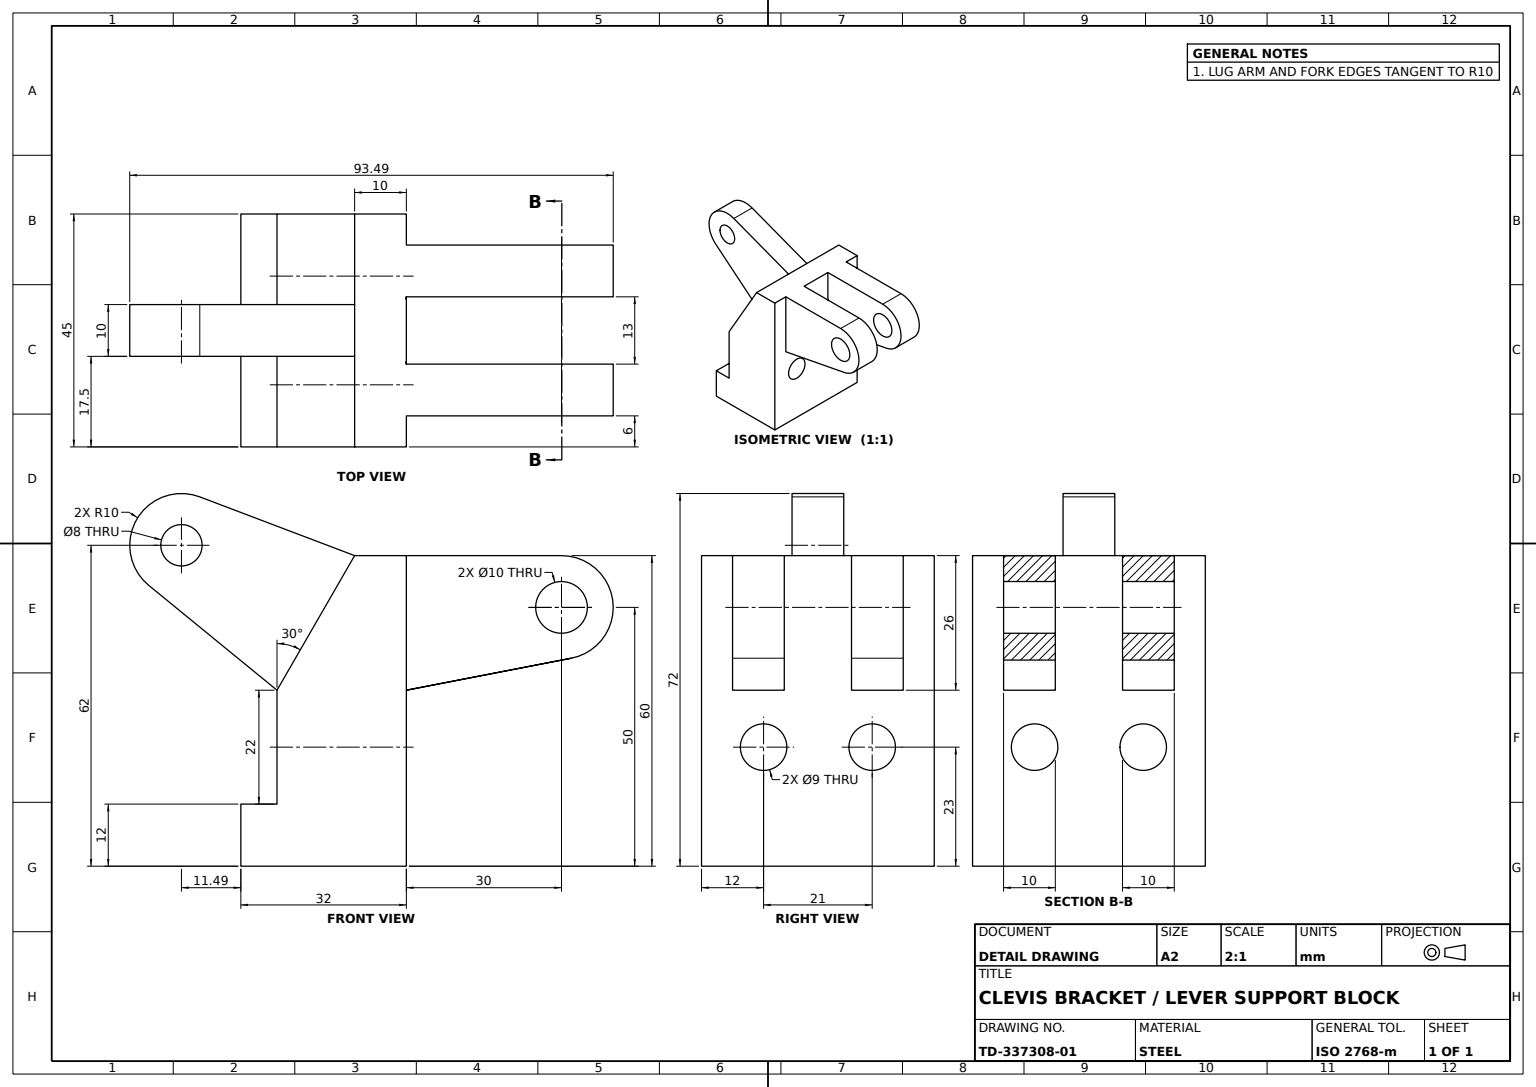
from build123d import *

# Parameters (mm, degrees)
BASE_BLOCK_DEPTH           = 22.5
LUG_ARM_SKETCH_R           = 4
LUG_ARM_DEPTH              = 5
SIDE_HOLE_9_REACH          = 82.629
SIDE_HOLE_SKETCH_R         = 4.5
CLEVIS_FORK_SKETCH_R       = 5
CLEVIS_FORK_DEPTH          = 45
CLEVIS_PIN_HOLE_SKETCH_W   = 40
CLEVIS_PIN_HOLE_SKETCH_H   = 6
CLEVIS_PIN_HOLE_SKETCH_H_2 = 13
CLEVIS_PIN_HOLES_6_DEPTH   = 84.468772351


with BuildPart() as part:
    # Base Block Profile Sketch → Base Block (new, symmetric)
    with BuildSketch(Plane.XY):
        Polygon((0, 0), (-32, 0), (-32, 12), (-25.011106999, 12), (-25.011106999, 34), (-10, 60), (0, 60), align=None)
    extrude(amount=BASE_BLOCK_DEPTH, both=True)

    # Lug Arm Sketch → Lug Arm (add, symmetric)
    with BuildSketch(Plane.XY):
        with BuildLine():
            Line((-25.011106999, 34), (-49.811828564, 54.254815308))
            ThreePointArc((-49.811828564, 54.254815308), (-52.146569651, 67), (-39.941545389, 71.350647253))
            Line((-39.941545389, 71.350647253), (-10, 60))
            Line((-10, 60), (-25.011106999, 34))
        make_face()
        with Locations((-43.486315613, 62)):
            Circle(LUG_ARM_SKETCH_R, mode=Mode.SUBTRACT)
    extrude(amount=LUG_ARM_DEPTH, both=True)

    # Side Hole Sketch → Side Hole Ø9 (cut, up to next)
    with BuildSketch(Plane.ZY.offset(25.011106999), mode=Mode.PRIVATE) as side_hole_9_sk1:
        with Locations((10.5, 23)):
            Circle(SIDE_HOLE_SKETCH_R)
    side_hole_9_tool1 = extrude(side_hole_9_sk1.sketch, amount=-SIDE_HOLE_9_REACH, mode=Mode.PRIVATE) & part.part
    # Side Hole Sketch → Side Hole Ø9 (cut, up to next)
    with BuildSketch(Plane.ZY.offset(25.011106999), mode=Mode.PRIVATE) as side_hole_9_sk2:
        with Locations((-10.5, 23)):
            Circle(SIDE_HOLE_SKETCH_R)
    side_hole_9_tool2 = extrude(side_hole_9_sk2.sketch, amount=-SIDE_HOLE_9_REACH, mode=Mode.PRIVATE) & part.part
    add(side_hole_9_tool1.solids().sort_by_distance((-25.011107, 23, 10.5))[0], mode=Mode.SUBTRACT)
    add(side_hole_9_tool2.solids().sort_by_distance((-25.011107, 23, -10.5))[0], mode=Mode.SUBTRACT)

    # Clevis Fork Sketch → Clevis Fork (add)
    with BuildSketch(Plane.XY.offset(22.5)):
        with BuildLine():
            Line((0, 60), (30, 60))
            ThreePointArc((30, 60), (39.954230484, 50.95566494), (31.902581816, 40.182659096))
            Line((31.902581816, 40.182659096), (0, 34))
            Line((0, 34), (0, 60))
        make_face()
        with Locations((30, 50)):
            Circle(CLEVIS_FORK_SKETCH_R, mode=Mode.SUBTRACT)
    extrude(amount=-CLEVIS_FORK_DEPTH)

    # Clevis Pin Hole Sketch → Clevis Pin Holes Ø6 (cut, through all)
    with BuildSketch(Plane(origin=(0, 60, 0), x_dir=(1, 0, 0), z_dir=(0, 1, 0))):
        with Locations((20, -19.5)):
            Rectangle(CLEVIS_PIN_HOLE_SKETCH_W, CLEVIS_PIN_HOLE_SKETCH_H)
        with Locations((20, 0)):
            Rectangle(CLEVIS_PIN_HOLE_SKETCH_W, CLEVIS_PIN_HOLE_SKETCH_H_2)
        with Locations((20, 19.5)):
            Rectangle(CLEVIS_PIN_HOLE_SKETCH_W, CLEVIS_PIN_HOLE_SKETCH_H)
    extrude(amount=-CLEVIS_PIN_HOLES_6_DEPTH, mode=Mode.SUBTRACT)


solid = part.part
